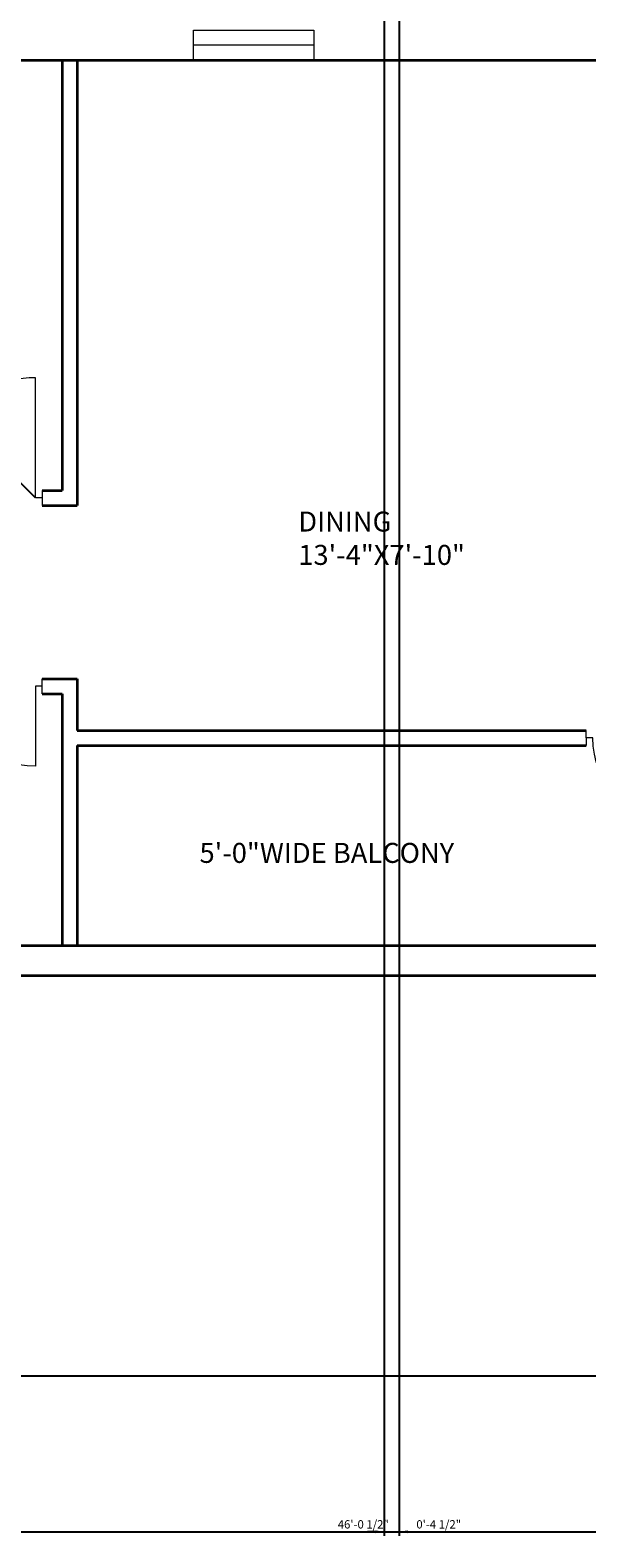
# Model space of a CAD drawing. Units: inches. Extents: x 3257 to 4085, y -12 to 956.
# Tile 2 of 6: x 3588 to 3755, y -12 to 441. Entities that reach past the tile are written whole.
import ezdxf

# ---------------------------------------------------------------- set-up
doc = ezdxf.new("R2010")
doc.units = ezdxf.units.IN
for name, color, linetype, lineweight in [('A-ANNO-DIMS', 2, 'Continuous', 18), ('A-AREA-IDEN', 7, 'Continuous', 18), ('A-DOOR', 3, 'Continuous', 18), ('A-GLAZ', 4, 'Continuous', 18), ('A-WALL', 7, 'Continuous', 35), ('C-PROP', 6, 'Continuous', 25)]:
    doc.layers.add(name, color=color, linetype=linetype, lineweight=lineweight)
doc.styles.get("Standard").update_dxf_attribs({"font": 'arial.ttf'})
doc.dimstyles.new('ISO-25', dxfattribs={"dimtxt": 2.5, "dimasz": 2.5, "dimexe": 1.25, "dimexo": 0.625, "dimtad": 1, "dimdec": 0, "dimlunit": 3, "dimtxsty": 'Standard', "dimcen": 2.5, "dimadec": 0, "dimazin": 0, "dimtfac": 1, "dimtdec": 0, "dimtmove": 0, "dimatfit": 3, "dimfxl": 1, "dimarcsym": 0})

# ---------------------------------------------------------------- blocks, each defined once
blk = doc.blocks.new('DOOR-SGL-24IN')
for p, q in [((2.25, 28), (0, 28)), ((2.25, 26), (2.25, 28)), ((2.25, 28), (4.5, 28)), ((2.25, 0), (2.25, 2)), ((2.25, 2), (26.25, 2)), ((4.5, 0), (0, 0))]:
    blk.add_line(p, q)
blk.add_arc((2.25, 2), 24, 0, 90)
blk = doc.blocks.new('WIN-36IN')
for p, q in [((0, 9), (36, 9)), ((0, 0), (0, 9)), ((36, 9), (36, 0)), ((0, 4.5), (36, 4.5)), ((36, 0), (0, 0))]:
    blk.add_line(p, q)
blk = doc.blocks.new('*D18')
at = {"layer": 'A-ANNO-DIMS', "color": 0, "lineweight": -2, "transparency": 16777216}
for p, q in [((3411.97, 156.38), (3411.97, -11.05)), ((3964.47, 156.38), (3964.47, -11.05)), ((3414.47, -9.8), (3961.97, -9.8))]:
    blk.add_line(p, q, dxfattribs=at)
at = {"layer": 'A-ANNO-DIMS', "color": 0, "transparency": 16777216}
for points in [[(3414.47, -9.38), (3414.47, -10.21), (3411.97, -9.8)], [(3961.97, -9.38), (3961.97, -10.21), (3964.47, -9.8)]]:
    blk.add_solid(points, dxfattribs=at)
at = {"layer": 'Defpoints', "color": 0, "transparency": 16777216}
for p in [(3411.97, 157), (3964.47, 157), (3964.47, -9.8)]:
    blk.add_point(p, dxfattribs=at)
at = {"layer": 'A-ANNO-DIMS', "color": 0, "transparency": 16777216, "insert": (3688.22, -7.88), "char_height": 2.5, "attachment_point": 5}
blk.add_mtext('46\'-0 1/2"', dxfattribs=at)
blk = doc.blocks.new('*D26')
at = {"layer": 'A-ANNO-DIMS', "color": 0, "lineweight": -2, "transparency": 16777216}
for p, q in [((3694.47, 710.38), (3694.47, -11.05)), ((3698.97, 710.38), (3698.97, -11.05)), ((3691.97, -9.8), (3689.47, -9.8)), ((3694.47, -9.8), (3698.97, -9.8)), ((3701.47, -9.8), (3717.69, -9.8))]:
    blk.add_line(p, q, dxfattribs=at)
at = {"layer": 'A-ANNO-DIMS', "color": 0, "transparency": 16777216}
for points in [[(3691.97, -9.38), (3691.97, -10.21), (3694.47, -9.8)], [(3701.47, -9.38), (3701.47, -10.21), (3698.97, -9.8)]]:
    blk.add_solid(points, dxfattribs=at)
at = {"layer": 'Defpoints', "color": 0, "transparency": 16777216}
for p in [(3694.47, 711), (3698.97, 711), (3698.97, -9.8)]:
    blk.add_point(p, dxfattribs=at)
at = {"layer": 'A-ANNO-DIMS', "color": 0, "transparency": 16777216, "insert": (3710.83, -7.88), "char_height": 2.5, "attachment_point": 5}
blk.add_mtext('0\'-4 1/2"', dxfattribs=at)
blk = doc.blocks.new('*D28')
at = {"layer": 'A-ANNO-DIMS', "color": 0, "lineweight": -2, "transparency": 16777216}
for p, q in [((3545.6, 344.62), (3562.74, 327.48)), ((3589.97, 300.25), (3564.51, 325.71))]:
    blk.add_line(p, q, dxfattribs=at)
at = {"layer": 'A-ANNO-DIMS', "color": 0, "transparency": 16777216}
blk.add_solid([(3563.04, 327.77), (3562.45, 327.18), (3564.51, 325.71)], dxfattribs=at)
at = {"layer": 'Defpoints', "color": 0, "transparency": 16777216}
for p in [(3564.51, 325.71), (3589.97, 300.25)]:
    blk.add_point(p, dxfattribs=at)
at = {"layer": 'A-ANNO-DIMS', "color": 0, "transparency": 16777216, "insert": (3550.58, 342.33), "char_height": 2.5, "attachment_point": 5, "rotation": 314.9996}
blk.add_mtext('R3\'-0"', dxfattribs=at)

msp = doc.modelspace()

# ---------------------------------------------------------------- linework, layer by layer
at = {"layer": 'A-DOOR'}
for p, q in [((3589.97, 300.25), (3589.97, 336.25)), ((3591.97, 300.25), (3589.97, 300.25)), ((3591.97, 302.5), (3591.97, 298))]:
    msp.add_line(p, q, dxfattribs=at)
msp.add_arc((3589.97, 300.25), 36, 90, 180, dxfattribs=at)
at = {"layer": 'A-WALL'}
for p, q in [((3420.97, 431.5), (3826.97, 431.5)), ((3597.97, 431.5), (3597.97, 302.5)), ((3602.47, 431.5), (3602.47, 298)), ((3591.97, 302.5), (3597.97, 302.5)), ((3591.97, 298), (3602.47, 298)), ((3591.97, 246), (3597.97, 246)), ((3597.97, 246), (3602.47, 246)), ((3602.47, 246), (3602.47, 230.5)), ((3591.97, 241.5), (3597.97, 241.5)), ((3597.97, 241.5), (3597.97, 166)), ((3602.47, 230.5), (3754.97, 230.5)), ((3602.47, 226), (3754.97, 226)), ((3602.47, 226), (3602.47, 166)), ((3420.97, 166), (3955.47, 166)), ((3411.97, 157), (3964.47, 157))]:
    msp.add_line(p, q, dxfattribs=at)
at = {"layer": 'C-PROP'}
msp.add_line((3411.97, 37), (3964.47, 37), dxfattribs=at)

# ---------------------------------------------------------------- block references
at = {"layer": 'A-DOOR', "extrusion": (0, 0, -1), "zscale": -1}
for p, rotation in [((-3591.97, 246), 269.9999999999996), ((-3782.97, 230.5), 269.9999999999985)]:
    msp.add_blockref('DOOR-SGL-24IN', p, dxfattribs=dict(at, rotation=rotation))
at = {"layer": 'A-GLAZ', "rotation": 180}
msp.add_blockref('WIN-36IN', (3673.37, 440.5), dxfattribs=at)

# ---------------------------------------------------------------- texts
at = {"layer": 'A-AREA-IDEN', "char_height": 6, "attachment_point": 1}
for s, insert in [('DINING\\P13\'-4"X7\'-10" ', (3668.74, 296.15)), ('5\'-0"WIDE BALCONY', (3639.14, 196.79))]:
    msp.add_mtext(s, dxfattribs=dict(at, insert=insert))

# ---------------------------------------------------------------- dimensions: what is measured, and where the dimension line sits
at = {"layer": 'A-ANNO-DIMS'}
for base, p1, p2, picture, middle in [((3698.97, -9.8), (3694.47, 711), (3698.97, 711), '*D26', (3710.83, -7.88)), ((3964.47, -9.8), (3411.97, 157), (3964.47, 157), '*D18', (3688.22, -7.88))]:
    dim = msp.add_linear_dim(base=base, p1=p1, p2=p2, dimstyle='ISO-25', override={"dimdec": 1, "dimlfac": 1, "dimrnd": 0, "dimzin": 1, "dimdsep": 46, "dimlunit": 4, "dimfrac": 2}, dxfattribs=at)
    dim.commit()
    dim.dimension.update_dxf_attribs({"geometry": picture, "text_midpoint": middle})
dim = msp.add_radius_dim(center=(3589.97, 300.25), mpoint=(3564.51, 325.71), dimstyle='ISO-25', override={"dimdec": 1, "dimlfac": 1, "dimrnd": 0, "dimzin": 1, "dimdsep": 46, "dimlunit": 4, "dimfrac": 2}, dxfattribs=at)
dim.commit()
dim.dimension.update_dxf_attribs({"geometry": '*D28', "text_midpoint": (3549.24, 340.98), "dimtype": 164})

doc.saveas('drawing.dxf')
